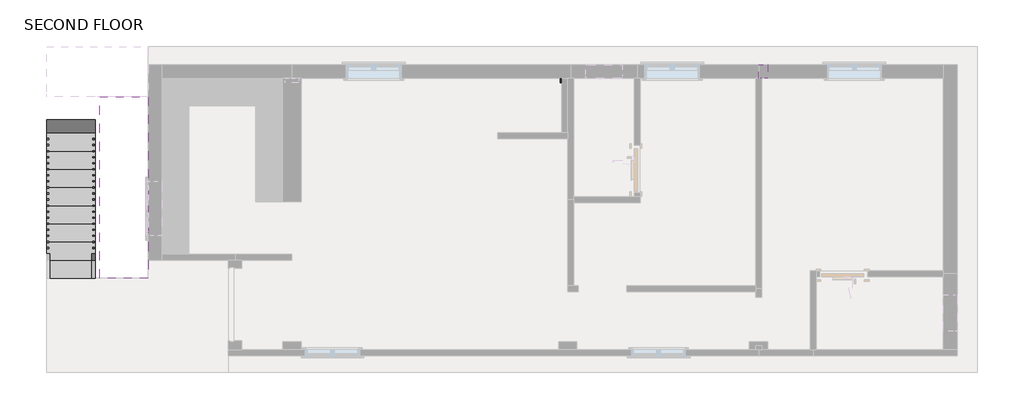
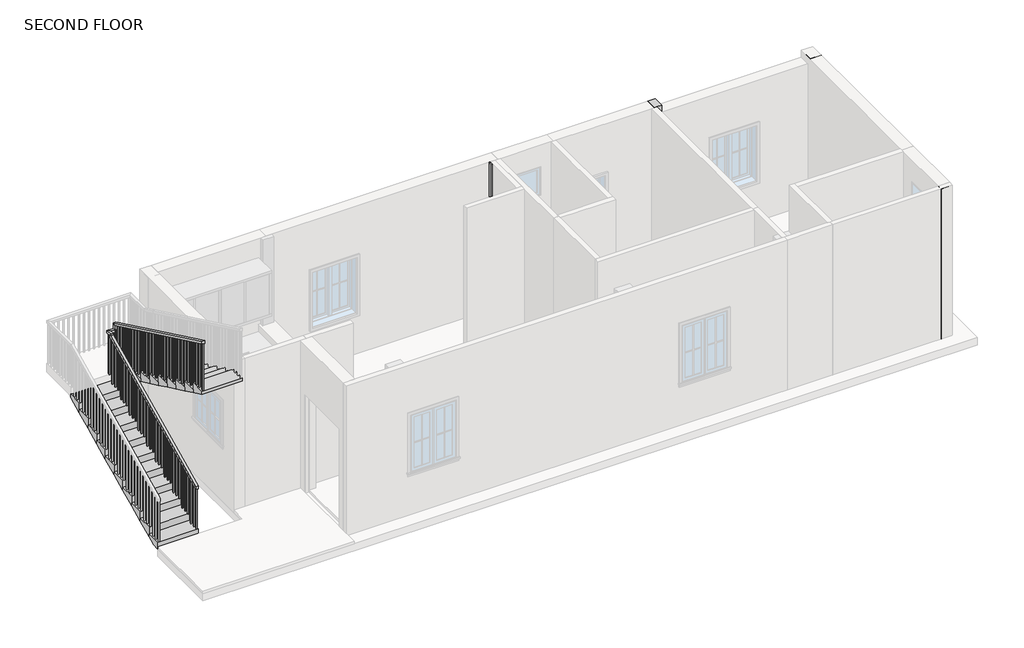
# One storey, part 2 of 3: 4 columns, 2 stair flights, 1 railing.
"""IFC4 building model written with IfcOpenShell, lengths in millimetres."""

from ifc_helpers import new_model, si_unit, frame, origin, place, context, project, spatial, polyline, outline, extrude, faceted_brep, element, save

model = new_model("IFC4")

# Units and contexts
model_context = context("Model", 3, world=origin())
ifc_project = project(units=[si_unit("LENGTHUNIT", "METRE", prefix="MILLI")], contexts=[model_context])

# Site, building, storey
site = spatial("IfcSite", under=ifc_project)
building = spatial("IfcBuilding", under=site)
storey = spatial("IfcBuildingStorey", under=building, Name="SECOND FLOOR", Elevation=6400.8)

# Columns
placement = place(None, origin())
element("IfcColumn", 1, ObjectType="Rectangular Column : 9\" X 12\"", at=placement, inside=storey, context=model_context, shape_type="Brep", body=[
    faceted_brep([(8641.6408773, 5102.5642852, 6400.8), (8870.2408773, 5102.5642852, 6400.8), (8870.2408773, 4797.7642852, 6400.8), (8641.6408773, 4797.7642852, 6400.8), (8641.6408773, 4873.9642852, 6400.8), (8641.6408773, 5102.5642852, 9601.2), (8870.2408773, 5102.5642852, 9601.2), (8641.6408773, 5102.5642852, 9448.8), (8870.2408773, 4797.7642852, 9601.2), (8641.6408773, 4797.7642852, 9601.2)], [[[0, 1, 2, 3, 4]], [[5, 6, 1, 0, 7]], [[6, 8, 2, 1]], [[8, 9, 3, 2]], [[9, 5, 7, 0, 4, 3]], [[5, 9, 8, 6]]]),
])
element("IfcColumn", 2, ObjectType="Rectangular Column : 9\" X 12\"", at=placement, inside=storey, context=model_context, shape_type="Brep", body=[
    faceted_brep([(5695.2408773, 5102.5642852, 9601.2), (5695.2408773, 5102.5642852, 9448.8), (5542.8408773, 5102.5642852, 9448.8), (5542.8408773, 5102.5642852, 9601.2), (5695.2408773, 4873.9642852, 9601.2), (5695.2408773, 4873.9642852, 9448.8), (5593.6408773, 4873.9642852, 9601.2), (5542.8408773, 4873.9642852, 9601.2), (5542.8408773, 4873.9642852, 9448.8)], [[[0, 1, 2, 3]], [[0, 4, 5, 1]], [[5, 4, 6, 7, 8]], [[4, 0, 3, 7, 6]], [[2, 1, 5, 8]], [[3, 2, 8, 7]]]),
])
element("IfcColumn", 3, ObjectType="Rectangular Column : 9\" X 12\"", at=placement, inside=storey, context=model_context, shape_type="SweptSolid", body=[
    extrude(outline(polyline([(2240.8408773, 4797.7642852), (2215.4408773, 4797.7642852), (2215.4408773, 4873.9642852), (2240.8408773, 4873.9642852), (2240.8408773, 4797.7642852)])), frame((0.0, 0.0, 6400.8), z_axis=(0.0, 0.0, 1.0), x_axis=(1.0, 0.0, 0.0)), (0.0, 0.0, 1.0), 3200.4),
])
element("IfcColumn", 4, ObjectType="Rectangular Column : 9\" X 12\"", at=placement, inside=storey, context=model_context, shape_type="SweptSolid", body=[
    extrude(outline(polyline([(8870.2408773, 225.7642852), (8641.6408773, 225.7642852), (8641.6408773, 327.3642852), (8870.2408773, 327.3642852), (8870.2408773, 225.7642852)])), frame((0.0, 0.0, 6400.8), z_axis=(0.0, 0.0, 1.0), x_axis=(1.0, 0.0, 0.0)), (0.0, 0.0, 1.0), 3200.4),
])

# Railing
element("IfcRailing", 5, ObjectType="Handrail - Rectangular", at=placement, inside=storey, context=model_context, shape_type="SolidModel", body=[
    faceted_brep([(-5633.1591227, 1521.1642852, 7460.6727273), (-5633.1591227, 1521.1642852, 7404.3834559), (-5582.3591227, 1521.1642852, 7404.3834559), (-5582.3591227, 1521.1642852, 7460.6727273), (-5633.1591227, 4492.9642852, 8879.0318182), (-5633.1591227, 4543.7642852, 8846.9880014), (-5582.3591227, 4543.7642852, 8846.9880014), (-5582.3591227, 4492.9642852, 8879.0318182), (-5633.1591227, 4492.9642852, 8915.4), (-5633.1591227, 4543.7642852, 8864.6), (-5582.3591227, 4543.7642852, 8864.6), (-5582.3591227, 4492.9642852, 8915.4), (-5633.1591227, 4619.9642852, 8915.4), (-5633.1591227, 4619.9642852, 8864.6), (-5582.3591227, 4569.1642852, 8864.6), (-5582.3591227, 4569.1642852, 8915.4), (-5506.1591227, 4619.9642852, 8915.4), (-5506.1591227, 4619.9642852, 8864.6), (-5506.1591227, 4569.1642852, 8864.6), (-5506.1591227, 4569.1642852, 8915.4), (-5480.7591227, 4619.9642852, 8915.4), (-5480.7591227, 4569.1642852, 8915.4), (-5480.7591227, 4569.1642852, 8864.6), (-5480.7591227, 4619.9642852, 8864.6)], [[[0, 1, 2, 3]], [[1, 0, 4, 5]], [[2, 1, 5, 6]], [[3, 2, 6, 7]], [[0, 3, 7, 4]], [[5, 4, 8, 9]], [[6, 5, 9, 10]], [[7, 6, 10, 11]], [[4, 7, 11, 8]], [[9, 8, 12, 13]], [[10, 9, 13, 14]], [[11, 10, 14, 15]], [[8, 11, 15, 12]], [[13, 12, 16, 17]], [[14, 13, 17, 18]], [[15, 14, 18, 19]], [[12, 15, 19, 16]], [[20, 21, 22, 23]], [[17, 16, 20, 23]], [[18, 17, 23, 22]], [[19, 18, 22, 21]], [[16, 19, 21, 20]]]),
    faceted_brep([(-5506.1591227, 4619.9642852, 8915.4), (-5455.3591227, 4619.9642852, 8864.6), (-5455.3591227, 4569.1642852, 8864.6), (-5506.1591227, 4569.1642852, 8915.4), (-5506.1591227, 4619.9642852, 9036.6272727), (-5506.1591227, 4569.1642852, 9004.5834559), (-5455.3591227, 4569.1642852, 9004.5834559), (-5455.3591227, 4619.9642852, 9036.6272727)], [[[0, 1, 2, 3]], [[4, 5, 6, 7]], [[1, 0, 4, 7]], [[2, 1, 7, 6]], [[3, 2, 6, 5]], [[0, 3, 5, 4]]]),
    faceted_brep([(-5455.3591227, 4619.9642852, 9036.6272727), (-5455.3591227, 4569.1642852, 9004.5834559), (-5506.1591227, 4569.1642852, 9004.5834559), (-5506.1591227, 4619.9642852, 9036.6272727), (-5455.3591227, 1521.1642852, 10515.6), (-5506.1591227, 1521.1642852, 10515.6), (-5506.1591227, 1521.1642852, 10459.3107287), (-5455.3591227, 1521.1642852, 10459.3107287)], [[[0, 1, 2, 3]], [[4, 5, 6, 7]], [[1, 0, 4, 7]], [[2, 1, 7, 6]], [[3, 2, 6, 5]], [[0, 3, 5, 4]]]),
    extrude(outline(polyline([(1537.0392852, 10451.7340241), (1556.0892852, 10442.6419787), (1556.0892852, 9455.7272727), (1537.0392852, 9455.7272727), (1537.0392852, 10451.7340241)])), frame((-5490.2841227, 0.0, 0.0), z_axis=(1.0, 0.0, 0.0), x_axis=(0.0, 1.0, 0.0)), (0.0, 0.0, 1.0), 19.05),
    extrude(outline(polyline([(1638.6392852, 10403.243115), (1657.6892852, 10394.1510696), (1657.6892852, 9455.7272727), (1638.6392852, 9455.7272727), (1638.6392852, 10403.243115)])), frame((-5490.2841227, 0.0, 0.0), z_axis=(1.0, 0.0, 0.0), x_axis=(0.0, 1.0, 0.0)), (0.0, 0.0, 1.0), 19.05),
    extrude(outline(polyline([(1740.2392852, 10354.7522059), (1759.2892852, 10345.6601605), (1759.2892852, 9455.7272727), (1740.2392852, 9455.7272727), (1740.2392852, 10354.7522059)])), frame((-5490.2841227, 0.0, 0.0), z_axis=(1.0, 0.0, 0.0), x_axis=(0.0, 1.0, 0.0)), (0.0, 0.0, 1.0), 19.05),
    extrude(outline(polyline([(1841.8392852, 10306.2612969), (1860.8892852, 10297.1692514), (1860.8892852, 9310.2545455), (1841.8392852, 9310.2545455), (1841.8392852, 10306.2612969)])), frame((-5490.2841227, 0.0, 0.0), z_axis=(1.0, 0.0, 0.0), x_axis=(0.0, 1.0, 0.0)), (0.0, 0.0, 1.0), 19.05),
    extrude(outline(polyline([(1943.4392852, 10257.7703878), (1962.4892852, 10248.6783423), (1962.4892852, 9310.2545455), (1943.4392852, 9310.2545455), (1943.4392852, 10257.7703878)])), frame((-5490.2841227, 0.0, 0.0), z_axis=(1.0, 0.0, 0.0), x_axis=(0.0, 1.0, 0.0)), (0.0, 0.0, 1.0), 19.05),
    extrude(outline(polyline([(2045.0392852, 10209.2794787), (2064.0892852, 10200.1874332), (2064.0892852, 9310.2545455), (2045.0392852, 9310.2545455), (2045.0392852, 10209.2794787)])), frame((-5490.2841227, 0.0, 0.0), z_axis=(1.0, 0.0, 0.0), x_axis=(0.0, 1.0, 0.0)), (0.0, 0.0, 1.0), 19.05),
    extrude(outline(polyline([(2146.6392852, 10160.7885696), (2165.6892852, 10151.6965241), (2165.6892852, 9164.7818182), (2146.6392852, 9164.7818182), (2146.6392852, 10160.7885696)])), frame((-5490.2841227, 0.0, 0.0), z_axis=(1.0, 0.0, 0.0), x_axis=(0.0, 1.0, 0.0)), (0.0, 0.0, 1.0), 19.05),
    extrude(outline(polyline([(2248.2392852, 10112.2976605), (2267.2892852, 10103.205615), (2267.2892852, 9164.7818182), (2248.2392852, 9164.7818182), (2248.2392852, 10112.2976605)])), frame((-5490.2841227, 0.0, 0.0), z_axis=(1.0, 0.0, 0.0), x_axis=(0.0, 1.0, 0.0)), (0.0, 0.0, 1.0), 19.05),
    extrude(outline(polyline([(2349.8392852, 10063.8067514), (2368.8892852, 10054.7147059), (2368.8892852, 9164.7818182), (2349.8392852, 9164.7818182), (2349.8392852, 10063.8067514)])), frame((-5490.2841227, 0.0, 0.0), z_axis=(1.0, 0.0, 0.0), x_axis=(0.0, 1.0, 0.0)), (0.0, 0.0, 1.0), 19.05),
    extrude(outline(polyline([(2451.4392852, 10015.3158423), (2470.4892852, 10006.2237969), (2470.4892852, 9019.3090909), (2451.4392852, 9019.3090909), (2451.4392852, 10015.3158423)])), frame((-5490.2841227, 0.0, 0.0), z_axis=(1.0, 0.0, 0.0), x_axis=(0.0, 1.0, 0.0)), (0.0, 0.0, 1.0), 19.05),
    extrude(outline(polyline([(2553.0392852, 9966.8249332), (2572.0892852, 9957.7328878), (2572.0892852, 9019.3090909), (2553.0392852, 9019.3090909), (2553.0392852, 9966.8249332)])), frame((-5490.2841227, 0.0, 0.0), z_axis=(1.0, 0.0, 0.0), x_axis=(0.0, 1.0, 0.0)), (0.0, 0.0, 1.0), 19.05),
    extrude(outline(polyline([(2654.6392852, 9918.3340241), (2673.6892852, 9909.2419787), (2673.6892852, 9019.3090909), (2654.6392852, 9019.3090909), (2654.6392852, 9918.3340241)])), frame((-5490.2841227, 0.0, 0.0), z_axis=(1.0, 0.0, 0.0), x_axis=(0.0, 1.0, 0.0)), (0.0, 0.0, 1.0), 19.05),
    extrude(outline(polyline([(2756.2392852, 9869.843115), (2775.2892852, 9860.7510696), (2775.2892852, 8873.8363636), (2756.2392852, 8873.8363636), (2756.2392852, 9869.843115)])), frame((-5490.2841227, 0.0, 0.0), z_axis=(1.0, 0.0, 0.0), x_axis=(0.0, 1.0, 0.0)), (0.0, 0.0, 1.0), 19.05),
    extrude(outline(polyline([(2857.8392852, 9821.3522059), (2876.8892852, 9812.2601605), (2876.8892852, 8873.8363636), (2857.8392852, 8873.8363636), (2857.8392852, 9821.3522059)])), frame((-5490.2841227, 0.0, 0.0), z_axis=(1.0, 0.0, 0.0), x_axis=(0.0, 1.0, 0.0)), (0.0, 0.0, 1.0), 19.05),
    extrude(outline(polyline([(2959.4392852, 9772.8612969), (2978.4892852, 9763.7692514), (2978.4892852, 8873.8363636), (2959.4392852, 8873.8363636), (2959.4392852, 9772.8612969)])), frame((-5490.2841227, 0.0, 0.0), z_axis=(1.0, 0.0, 0.0), x_axis=(0.0, 1.0, 0.0)), (0.0, 0.0, 1.0), 19.05),
    extrude(outline(polyline([(3061.0392852, 9724.3703878), (3080.0892852, 9715.2783423), (3080.0892852, 8728.3636364), (3061.0392852, 8728.3636364), (3061.0392852, 9724.3703878)])), frame((-5490.2841227, 0.0, 0.0), z_axis=(1.0, 0.0, 0.0), x_axis=(0.0, 1.0, 0.0)), (0.0, 0.0, 1.0), 19.05),
    extrude(outline(polyline([(3162.6392852, 9675.8794787), (3181.6892852, 9666.7874332), (3181.6892852, 8728.3636364), (3162.6392852, 8728.3636364), (3162.6392852, 9675.8794787)])), frame((-5490.2841227, 0.0, 0.0), z_axis=(1.0, 0.0, 0.0), x_axis=(0.0, 1.0, 0.0)), (0.0, 0.0, 1.0), 19.05),
    extrude(outline(polyline([(3264.2392852, 9627.3885696), (3283.2892852, 9618.2965241), (3283.2892852, 8728.3636364), (3264.2392852, 8728.3636364), (3264.2392852, 9627.3885696)])), frame((-5490.2841227, 0.0, 0.0), z_axis=(1.0, 0.0, 0.0), x_axis=(0.0, 1.0, 0.0)), (0.0, 0.0, 1.0), 19.05),
    extrude(outline(polyline([(3365.8392852, 9578.8976605), (3384.8892852, 9569.805615), (3384.8892852, 8582.8909091), (3365.8392852, 8582.8909091), (3365.8392852, 9578.8976605)])), frame((-5490.2841227, 0.0, 0.0), z_axis=(1.0, 0.0, 0.0), x_axis=(0.0, 1.0, 0.0)), (0.0, 0.0, 1.0), 19.05),
    extrude(outline(polyline([(3467.4392852, 9530.4067514), (3486.4892852, 9521.3147059), (3486.4892852, 8582.8909091), (3467.4392852, 8582.8909091), (3467.4392852, 9530.4067514)])), frame((-5490.2841227, 0.0, 0.0), z_axis=(1.0, 0.0, 0.0), x_axis=(0.0, 1.0, 0.0)), (0.0, 0.0, 1.0), 19.05),
    extrude(outline(polyline([(3569.0392852, 9481.9158423), (3588.0892852, 9472.8237969), (3588.0892852, 8582.8909091), (3569.0392852, 8582.8909091), (3569.0392852, 9481.9158423)])), frame((-5490.2841227, 0.0, 0.0), z_axis=(1.0, 0.0, 0.0), x_axis=(0.0, 1.0, 0.0)), (0.0, 0.0, 1.0), 19.05),
    extrude(outline(polyline([(3670.6392852, 9433.4249332), (3689.6892852, 9424.3328878), (3689.6892852, 8437.4181818), (3670.6392852, 8437.4181818), (3670.6392852, 9433.4249332)])), frame((-5490.2841227, 0.0, 0.0), z_axis=(1.0, 0.0, 0.0), x_axis=(0.0, 1.0, 0.0)), (0.0, 0.0, 1.0), 19.05),
    extrude(outline(polyline([(3772.2392852, 9384.9340241), (3791.2892852, 9375.8419787), (3791.2892852, 8437.4181818), (3772.2392852, 8437.4181818), (3772.2392852, 9384.9340241)])), frame((-5490.2841227, 0.0, 0.0), z_axis=(1.0, 0.0, 0.0), x_axis=(0.0, 1.0, 0.0)), (0.0, 0.0, 1.0), 19.05),
    extrude(outline(polyline([(3873.8392852, 9336.443115), (3892.8892852, 9327.3510696), (3892.8892852, 8437.4181818), (3873.8392852, 8437.4181818), (3873.8392852, 9336.443115)])), frame((-5490.2841227, 0.0, 0.0), z_axis=(1.0, 0.0, 0.0), x_axis=(0.0, 1.0, 0.0)), (0.0, 0.0, 1.0), 19.05),
    extrude(outline(polyline([(3975.4392852, 9287.9522059), (3994.4892852, 9278.8601605), (3994.4892852, 8291.9454545), (3975.4392852, 8291.9454545), (3975.4392852, 9287.9522059)])), frame((-5490.2841227, 0.0, 0.0), z_axis=(1.0, 0.0, 0.0), x_axis=(0.0, 1.0, 0.0)), (0.0, 0.0, 1.0), 19.05),
    extrude(outline(polyline([(4077.0392852, 9239.4612969), (4096.0892852, 9230.3692514), (4096.0892852, 8291.9454545), (4077.0392852, 8291.9454545), (4077.0392852, 9239.4612969)])), frame((-5490.2841227, 0.0, 0.0), z_axis=(1.0, 0.0, 0.0), x_axis=(0.0, 1.0, 0.0)), (0.0, 0.0, 1.0), 19.05),
    extrude(outline(polyline([(4178.6392852, 9190.9703878), (4197.6892852, 9181.8783423), (4197.6892852, 8291.9454545), (4178.6392852, 8291.9454545), (4178.6392852, 9190.9703878)])), frame((-5490.2841227, 0.0, 0.0), z_axis=(1.0, 0.0, 0.0), x_axis=(0.0, 1.0, 0.0)), (0.0, 0.0, 1.0), 19.05),
    extrude(outline(polyline([(4280.2392852, 9142.4794787), (4299.2892852, 9133.3874332), (4299.2892852, 8146.4727273), (4280.2392852, 8146.4727273), (4280.2392852, 9142.4794787)])), frame((-5490.2841227, 0.0, 0.0), z_axis=(1.0, 0.0, 0.0), x_axis=(0.0, 1.0, 0.0)), (0.0, 0.0, 1.0), 19.05),
    extrude(outline(polyline([(4381.8392852, 9093.9885696), (4400.8892852, 9084.8965241), (4400.8892852, 8146.4727273), (4381.8392852, 8146.4727273), (4381.8392852, 9093.9885696)])), frame((-5490.2841227, 0.0, 0.0), z_axis=(1.0, 0.0, 0.0), x_axis=(0.0, 1.0, 0.0)), (0.0, 0.0, 1.0), 19.05),
    extrude(outline(polyline([(4483.4392852, 9045.4976605), (4502.4892852, 9036.405615), (4502.4892852, 8146.4727273), (4483.4392852, 8146.4727273), (4483.4392852, 9045.4976605)])), frame((-5490.2841227, 0.0, 0.0), z_axis=(1.0, 0.0, 0.0), x_axis=(0.0, 1.0, 0.0)), (0.0, 0.0, 1.0), 19.05),
    extrude(outline(polyline([(-5515.6841227, 4585.0392852), (-5515.6841227, 4604.0892852), (-5496.6341227, 4604.0892852), (-5496.6341227, 4585.0392852), (-5515.6841227, 4585.0392852)])), frame((0.0, 0.0, 8001.0), z_axis=(0.0, 0.0, 1.0), x_axis=(1.0, 0.0, 0.0)), (0.0, 0.0, 1.0), 863.6),
    extrude(outline(polyline([(-5598.2341227, 4559.6392852), (-5617.2841227, 4559.6392852), (-5617.2841227, 4578.6892852), (-5598.2341227, 4578.6892852), (-5598.2341227, 4559.6392852)])), frame((0.0, 0.0, 8001.0), z_axis=(0.0, 0.0, 1.0), x_axis=(1.0, 0.0, 0.0)), (0.0, 0.0, 1.0), 863.6),
    extrude(outline(polyline([(4458.0392852, 8806.0737969), (4477.0892852, 8815.1658423), (4477.0892852, 7855.5272727), (4458.0392852, 7855.5272727), (4458.0392852, 8806.0737969)])), frame((-5617.2841227, 0.0, 0.0), z_axis=(1.0, 0.0, 0.0), x_axis=(0.0, 1.0, 0.0)), (0.0, 0.0, 1.0), 19.05),
    extrude(outline(polyline([(4356.4392852, 8757.5828878), (4375.4892852, 8766.6749332), (4375.4892852, 7855.5272727), (4356.4392852, 7855.5272727), (4356.4392852, 8757.5828878)])), frame((-5617.2841227, 0.0, 0.0), z_axis=(1.0, 0.0, 0.0), x_axis=(0.0, 1.0, 0.0)), (0.0, 0.0, 1.0), 19.05),
    extrude(outline(polyline([(4254.8392852, 8709.0919787), (4273.8892852, 8718.1840241), (4273.8892852, 7855.5272727), (4254.8392852, 7855.5272727), (4254.8392852, 8709.0919787)])), frame((-5617.2841227, 0.0, 0.0), z_axis=(1.0, 0.0, 0.0), x_axis=(0.0, 1.0, 0.0)), (0.0, 0.0, 1.0), 19.05),
    extrude(outline(polyline([(4153.2392852, 8660.6010696), (4172.2892852, 8669.693115), (4172.2892852, 7710.0545455), (4153.2392852, 7710.0545455), (4153.2392852, 8660.6010696)])), frame((-5617.2841227, 0.0, 0.0), z_axis=(1.0, 0.0, 0.0), x_axis=(0.0, 1.0, 0.0)), (0.0, 0.0, 1.0), 19.05),
    extrude(outline(polyline([(4051.6392852, 8612.1101605), (4070.6892852, 8621.2022059), (4070.6892852, 7710.0545455), (4051.6392852, 7710.0545455), (4051.6392852, 8612.1101605)])), frame((-5617.2841227, 0.0, 0.0), z_axis=(1.0, 0.0, 0.0), x_axis=(0.0, 1.0, 0.0)), (0.0, 0.0, 1.0), 19.05),
    extrude(outline(polyline([(3950.0392852, 8563.6192514), (3969.0892852, 8572.7112969), (3969.0892852, 7710.0545455), (3950.0392852, 7710.0545455), (3950.0392852, 8563.6192514)])), frame((-5617.2841227, 0.0, 0.0), z_axis=(1.0, 0.0, 0.0), x_axis=(0.0, 1.0, 0.0)), (0.0, 0.0, 1.0), 19.05),
    extrude(outline(polyline([(3848.4392852, 8515.1283423), (3867.4892852, 8524.2203878), (3867.4892852, 7564.5818182), (3848.4392852, 7564.5818182), (3848.4392852, 8515.1283423)])), frame((-5617.2841227, 0.0, 0.0), z_axis=(1.0, 0.0, 0.0), x_axis=(0.0, 1.0, 0.0)), (0.0, 0.0, 1.0), 19.05),
    extrude(outline(polyline([(3746.8392852, 8466.6374332), (3765.8892852, 8475.7294787), (3765.8892852, 7564.5818182), (3746.8392852, 7564.5818182), (3746.8392852, 8466.6374332)])), frame((-5617.2841227, 0.0, 0.0), z_axis=(1.0, 0.0, 0.0), x_axis=(0.0, 1.0, 0.0)), (0.0, 0.0, 1.0), 19.05),
    extrude(outline(polyline([(3645.2392852, 8418.1465241), (3664.2892852, 8427.2385696), (3664.2892852, 7564.5818182), (3645.2392852, 7564.5818182), (3645.2392852, 8418.1465241)])), frame((-5617.2841227, 0.0, 0.0), z_axis=(1.0, 0.0, 0.0), x_axis=(0.0, 1.0, 0.0)), (0.0, 0.0, 1.0), 19.05),
    extrude(outline(polyline([(3543.6392852, 8369.655615), (3562.6892852, 8378.7476605), (3562.6892852, 7419.1090909), (3543.6392852, 7419.1090909), (3543.6392852, 8369.655615)])), frame((-5617.2841227, 0.0, 0.0), z_axis=(1.0, 0.0, 0.0), x_axis=(0.0, 1.0, 0.0)), (0.0, 0.0, 1.0), 19.05),
    extrude(outline(polyline([(3442.0392852, 8321.1647059), (3461.0892852, 8330.2567514), (3461.0892852, 7419.1090909), (3442.0392852, 7419.1090909), (3442.0392852, 8321.1647059)])), frame((-5617.2841227, 0.0, 0.0), z_axis=(1.0, 0.0, 0.0), x_axis=(0.0, 1.0, 0.0)), (0.0, 0.0, 1.0), 19.05),
    extrude(outline(polyline([(3340.4392852, 8272.6737969), (3359.4892852, 8281.7658423), (3359.4892852, 7419.1090909), (3340.4392852, 7419.1090909), (3340.4392852, 8272.6737969)])), frame((-5617.2841227, 0.0, 0.0), z_axis=(1.0, 0.0, 0.0), x_axis=(0.0, 1.0, 0.0)), (0.0, 0.0, 1.0), 19.05),
    extrude(outline(polyline([(3238.8392852, 8224.1828878), (3257.8892852, 8233.2749332), (3257.8892852, 7273.6363636), (3238.8392852, 7273.6363636), (3238.8392852, 8224.1828878)])), frame((-5617.2841227, 0.0, 0.0), z_axis=(1.0, 0.0, 0.0), x_axis=(0.0, 1.0, 0.0)), (0.0, 0.0, 1.0), 19.05),
    extrude(outline(polyline([(3137.2392852, 8175.6919787), (3156.2892852, 8184.7840241), (3156.2892852, 7273.6363636), (3137.2392852, 7273.6363636), (3137.2392852, 8175.6919787)])), frame((-5617.2841227, 0.0, 0.0), z_axis=(1.0, 0.0, 0.0), x_axis=(0.0, 1.0, 0.0)), (0.0, 0.0, 1.0), 19.05),
    extrude(outline(polyline([(3035.6392852, 8127.2010696), (3054.6892852, 8136.293115), (3054.6892852, 7273.6363636), (3035.6392852, 7273.6363636), (3035.6392852, 8127.2010696)])), frame((-5617.2841227, 0.0, 0.0), z_axis=(1.0, 0.0, 0.0), x_axis=(0.0, 1.0, 0.0)), (0.0, 0.0, 1.0), 19.05),
    extrude(outline(polyline([(2934.0392852, 8078.7101605), (2953.0892852, 8087.8022059), (2953.0892852, 7128.1636364), (2934.0392852, 7128.1636364), (2934.0392852, 8078.7101605)])), frame((-5617.2841227, 0.0, 0.0), z_axis=(1.0, 0.0, 0.0), x_axis=(0.0, 1.0, 0.0)), (0.0, 0.0, 1.0), 19.05),
    extrude(outline(polyline([(2832.4392852, 8030.2192514), (2851.4892852, 8039.3112969), (2851.4892852, 7128.1636364), (2832.4392852, 7128.1636364), (2832.4392852, 8030.2192514)])), frame((-5617.2841227, 0.0, 0.0), z_axis=(1.0, 0.0, 0.0), x_axis=(0.0, 1.0, 0.0)), (0.0, 0.0, 1.0), 19.05),
    extrude(outline(polyline([(2730.8392852, 7981.7283423), (2749.8892852, 7990.8203878), (2749.8892852, 7128.1636364), (2730.8392852, 7128.1636364), (2730.8392852, 7981.7283423)])), frame((-5617.2841227, 0.0, 0.0), z_axis=(1.0, 0.0, 0.0), x_axis=(0.0, 1.0, 0.0)), (0.0, 0.0, 1.0), 19.05),
    extrude(outline(polyline([(2629.2392852, 7933.2374332), (2648.2892852, 7942.3294787), (2648.2892852, 6982.6909091), (2629.2392852, 6982.6909091), (2629.2392852, 7933.2374332)])), frame((-5617.2841227, 0.0, 0.0), z_axis=(1.0, 0.0, 0.0), x_axis=(0.0, 1.0, 0.0)), (0.0, 0.0, 1.0), 19.05),
    extrude(outline(polyline([(2527.6392852, 7884.7465241), (2546.6892852, 7893.8385696), (2546.6892852, 6982.6909091), (2527.6392852, 6982.6909091), (2527.6392852, 7884.7465241)])), frame((-5617.2841227, 0.0, 0.0), z_axis=(1.0, 0.0, 0.0), x_axis=(0.0, 1.0, 0.0)), (0.0, 0.0, 1.0), 19.05),
    extrude(outline(polyline([(2426.0392852, 7836.255615), (2445.0892852, 7845.3476605), (2445.0892852, 6982.6909091), (2426.0392852, 6982.6909091), (2426.0392852, 7836.255615)])), frame((-5617.2841227, 0.0, 0.0), z_axis=(1.0, 0.0, 0.0), x_axis=(0.0, 1.0, 0.0)), (0.0, 0.0, 1.0), 19.05),
    extrude(outline(polyline([(2324.4392852, 7787.7647059), (2343.4892852, 7796.8567514), (2343.4892852, 6837.2181818), (2324.4392852, 6837.2181818), (2324.4392852, 7787.7647059)])), frame((-5617.2841227, 0.0, 0.0), z_axis=(1.0, 0.0, 0.0), x_axis=(0.0, 1.0, 0.0)), (0.0, 0.0, 1.0), 19.05),
    extrude(outline(polyline([(2222.8392852, 7739.2737969), (2241.8892852, 7748.3658423), (2241.8892852, 6837.2181818), (2222.8392852, 6837.2181818), (2222.8392852, 7739.2737969)])), frame((-5617.2841227, 0.0, 0.0), z_axis=(1.0, 0.0, 0.0), x_axis=(0.0, 1.0, 0.0)), (0.0, 0.0, 1.0), 19.05),
    extrude(outline(polyline([(2121.2392852, 7690.7828878), (2140.2892852, 7699.8749332), (2140.2892852, 6837.2181818), (2121.2392852, 6837.2181818), (2121.2392852, 7690.7828878)])), frame((-5617.2841227, 0.0, 0.0), z_axis=(1.0, 0.0, 0.0), x_axis=(0.0, 1.0, 0.0)), (0.0, 0.0, 1.0), 19.05),
    extrude(outline(polyline([(2019.6392852, 7642.2919787), (2038.6892852, 7651.3840241), (2038.6892852, 6691.7454545), (2019.6392852, 6691.7454545), (2019.6392852, 7642.2919787)])), frame((-5617.2841227, 0.0, 0.0), z_axis=(1.0, 0.0, 0.0), x_axis=(0.0, 1.0, 0.0)), (0.0, 0.0, 1.0), 19.05),
    extrude(outline(polyline([(1918.0392852, 7593.8010696), (1937.0892852, 7602.893115), (1937.0892852, 6691.7454545), (1918.0392852, 6691.7454545), (1918.0392852, 7593.8010696)])), frame((-5617.2841227, 0.0, 0.0), z_axis=(1.0, 0.0, 0.0), x_axis=(0.0, 1.0, 0.0)), (0.0, 0.0, 1.0), 19.05),
    extrude(outline(polyline([(1816.4392852, 7545.3101605), (1835.4892852, 7554.4022059), (1835.4892852, 6691.7454545), (1816.4392852, 6691.7454545), (1816.4392852, 7545.3101605)])), frame((-5617.2841227, 0.0, 0.0), z_axis=(1.0, 0.0, 0.0), x_axis=(0.0, 1.0, 0.0)), (0.0, 0.0, 1.0), 19.05),
    extrude(outline(polyline([(1714.8392852, 7496.8192514), (1733.8892852, 7505.9112969), (1733.8892852, 6546.2727273), (1714.8392852, 6546.2727273), (1714.8392852, 7496.8192514)])), frame((-5617.2841227, 0.0, 0.0), z_axis=(1.0, 0.0, 0.0), x_axis=(0.0, 1.0, 0.0)), (0.0, 0.0, 1.0), 19.05),
    extrude(outline(polyline([(1613.2392852, 7448.3283423), (1632.2892852, 7457.4203878), (1632.2892852, 6546.2727273), (1613.2392852, 6546.2727273), (1613.2392852, 7448.3283423)])), frame((-5617.2841227, 0.0, 0.0), z_axis=(1.0, 0.0, 0.0), x_axis=(0.0, 1.0, 0.0)), (0.0, 0.0, 1.0), 19.05),
    extrude(outline(polyline([(-5490.2841227, 4585.0392852), (-5490.2841227, 4604.0892852), (-5471.2341227, 4604.0892852), (-5471.2341227, 4585.0392852), (-5490.2841227, 4585.0392852)])), frame((0.0, 0.0, 8001.0), z_axis=(0.0, 0.0, 1.0), x_axis=(1.0, 0.0, 0.0)), (0.0, 0.0, 1.0), 863.6),
    extrude(outline(polyline([(-5598.2341227, 4585.0392852), (-5617.2841227, 4585.0392852), (-5617.2841227, 4604.0892852), (-5598.2341227, 4604.0892852), (-5598.2341227, 4585.0392852)])), frame((0.0, 0.0, 8001.0), z_axis=(0.0, 0.0, 1.0), x_axis=(1.0, 0.0, 0.0)), (0.0, 0.0, 1.0), 863.6),
    extrude(outline(polyline([(1521.1642852, 10459.3107287), (1540.2142852, 10450.2186832), (1540.2142852, 9455.7272727), (1521.1642852, 9455.7272727), (1521.1642852, 10459.3107287)])), frame((-5490.2841227, 0.0, 0.0), z_axis=(1.0, 0.0, 0.0), x_axis=(0.0, 1.0, 0.0)), (0.0, 0.0, 1.0), 19.05),
    extrude(outline(polyline([(1521.1642852, 7404.3834559), (1540.2142852, 7413.4755014), (1540.2142852, 6546.2727273), (1521.1642852, 6546.2727273), (1521.1642852, 7404.3834559)])), frame((-5617.2841227, 0.0, 0.0), z_axis=(1.0, 0.0, 0.0), x_axis=(0.0, 1.0, 0.0)), (0.0, 0.0, 1.0), 19.05),
])

# Stair flights
element("IfcStairFlight", 6, ObjectType="3/4\" Nosing", at=placement, inside=storey, context=model_context, shape_type="Brep", body=[
    faceted_brep([(-6395.1591227, 1825.9642852, 6546.2727273), (-6395.1591227, 1521.1642852, 6546.2727273), (-5582.3591227, 1521.1642852, 6546.2727273), (-5582.3591227, 1825.9642852, 6546.2727273), (-6395.1591227, 1825.9642852, 6475.9111381), (-6395.1591227, 1668.5885672, 6400.8), (-6395.1591227, 1521.1642852, 6400.8), (-5582.3591227, 1521.1642852, 6400.8), (-5582.3591227, 1668.5885672, 6400.8), (-5582.3591227, 1825.9642852, 6475.9111381), (-6395.1591227, 2130.7642852, 6691.7454545), (-6395.1591227, 1825.9642852, 6691.7454545), (-5582.3591227, 1825.9642852, 6691.7454545), (-5582.3591227, 2130.7642852, 6691.7454545), (-6395.1591227, 2130.7642852, 6621.3838654), (-5582.3591227, 2130.7642852, 6621.3838654), (-6395.1591227, 2435.5642852, 6837.2181818), (-6395.1591227, 2130.7642852, 6837.2181818), (-5582.3591227, 2130.7642852, 6837.2181818), (-5582.3591227, 2435.5642852, 6837.2181818), (-6395.1591227, 2435.5642852, 6766.8565927), (-5582.3591227, 2435.5642852, 6766.8565927), (-6395.1591227, 2740.3642852, 6982.6909091), (-6395.1591227, 2435.5642852, 6982.6909091), (-5582.3591227, 2435.5642852, 6982.6909091), (-5582.3591227, 2740.3642852, 6982.6909091), (-6395.1591227, 2740.3642852, 6912.3293199), (-5582.3591227, 2740.3642852, 6912.3293199), (-6395.1591227, 3045.1642852, 7128.1636364), (-6395.1591227, 2740.3642852, 7128.1636364), (-5582.3591227, 2740.3642852, 7128.1636364), (-5582.3591227, 3045.1642852, 7128.1636364), (-6395.1591227, 3045.1642852, 7057.8020472), (-5582.3591227, 3045.1642852, 7057.8020472), (-6395.1591227, 3349.9642852, 7273.6363636), (-6395.1591227, 3045.1642852, 7273.6363636), (-5582.3591227, 3045.1642852, 7273.6363636), (-5582.3591227, 3349.9642852, 7273.6363636), (-6395.1591227, 3349.9642852, 7203.2747745), (-5582.3591227, 3349.9642852, 7203.2747745), (-6395.1591227, 3654.7642852, 7419.1090909), (-6395.1591227, 3349.9642852, 7419.1090909), (-5582.3591227, 3349.9642852, 7419.1090909), (-5582.3591227, 3654.7642852, 7419.1090909), (-6395.1591227, 3654.7642852, 7348.7475018), (-5582.3591227, 3654.7642852, 7348.7475018), (-6395.1591227, 3959.5642852, 7564.5818182), (-6395.1591227, 3654.7642852, 7564.5818182), (-5582.3591227, 3654.7642852, 7564.5818182), (-5582.3591227, 3959.5642852, 7564.5818182), (-6395.1591227, 3959.5642852, 7494.220229), (-5582.3591227, 3959.5642852, 7494.220229), (-6395.1591227, 4264.3642852, 7639.6929563), (-6395.1591227, 4569.1642852, 7785.1656836), (-5582.3591227, 4569.1642852, 7785.1656836), (-5582.3591227, 4264.3642852, 7639.6929563), (-6395.1591227, 4264.3642852, 7710.0545455), (-6395.1591227, 3959.5642852, 7710.0545455), (-5582.3591227, 3959.5642852, 7710.0545455), (-5582.3591227, 4264.3642852, 7710.0545455), (-6395.1591227, 4569.1642852, 7855.5272727), (-6395.1591227, 4264.3642852, 7855.5272727), (-5582.3591227, 4264.3642852, 7855.5272727), (-5582.3591227, 4569.1642852, 7855.5272727), (-5582.3591227, 4569.1642852, 7823.2)], [[[0, 1, 2, 3]], [[1, 0, 4, 5, 6]], [[2, 1, 6, 7]], [[3, 2, 7, 8, 9]], [[10, 11, 12, 13]], [[11, 10, 14, 4, 0]], [[0, 3, 12, 11]], [[13, 12, 3, 9, 15]], [[16, 17, 18, 19]], [[17, 16, 20, 14, 10]], [[10, 13, 18, 17]], [[19, 18, 13, 15, 21]], [[22, 23, 24, 25]], [[23, 22, 26, 20, 16]], [[16, 19, 24, 23]], [[25, 24, 19, 21, 27]], [[28, 29, 30, 31]], [[29, 28, 32, 26, 22]], [[22, 25, 30, 29]], [[31, 30, 25, 27, 33]], [[34, 35, 36, 37]], [[35, 34, 38, 32, 28]], [[28, 31, 36, 35]], [[37, 36, 31, 33, 39]], [[40, 41, 42, 43]], [[41, 40, 44, 38, 34]], [[34, 37, 42, 41]], [[43, 42, 37, 39, 45]], [[46, 47, 48, 49]], [[47, 46, 50, 44, 40]], [[40, 43, 48, 47]], [[49, 48, 43, 45, 51]], [[7, 6, 5, 8]], [[8, 5, 4, 14, 20, 26, 32, 38, 44, 50, 52, 53, 54, 55, 51, 45, 39, 33, 27, 21, 15, 9]], [[56, 57, 58, 59]], [[57, 56, 52, 50, 46]], [[46, 49, 58, 57]], [[59, 58, 49, 51, 55]], [[60, 61, 62, 63]], [[61, 60, 53, 52, 56]], [[56, 59, 62, 61]], [[63, 62, 59, 55, 54, 64]], [[60, 63, 64, 54, 53]]]),
])
element("IfcStairFlight", 7, ObjectType="3/4\" Nosing", at=placement, inside=storey, context=model_context, shape_type="Brep", body=[
    faceted_brep([(-4693.3591227, 4264.3642852, 8146.4727273), (-4693.3591227, 4569.1642852, 8146.4727273), (-5506.1591227, 4569.1642852, 8146.4727273), (-5506.1591227, 4264.3642852, 8146.4727273), (-4693.3591227, 4264.3642852, 8076.1111381), (-4693.3591227, 4569.1642852, 7930.6384108), (-4693.3591227, 4569.1642852, 8001.0), (-5506.1591227, 4569.1642852, 7930.6384108), (-5506.1591227, 4264.3642852, 8076.1111381), (-4693.3591227, 3959.5642852, 8291.9454545), (-4693.3591227, 4264.3642852, 8291.9454545), (-5506.1591227, 4264.3642852, 8291.9454545), (-5506.1591227, 3959.5642852, 8291.9454545), (-4693.3591227, 3959.5642852, 8221.5838654), (-5506.1591227, 3959.5642852, 8221.5838654), (-4693.3591227, 3654.7642852, 8437.4181818), (-4693.3591227, 3959.5642852, 8437.4181818), (-5506.1591227, 3959.5642852, 8437.4181818), (-5506.1591227, 3654.7642852, 8437.4181818), (-4693.3591227, 3654.7642852, 8367.0565927), (-5506.1591227, 3654.7642852, 8367.0565927), (-4693.3591227, 3349.9642852, 8582.8909091), (-4693.3591227, 3654.7642852, 8582.8909091), (-5506.1591227, 3654.7642852, 8582.8909091), (-5506.1591227, 3349.9642852, 8582.8909091), (-4693.3591227, 3349.9642852, 8512.5293199), (-5506.1591227, 3349.9642852, 8512.5293199), (-4693.3591227, 3045.1642852, 8728.3636364), (-4693.3591227, 3349.9642852, 8728.3636364), (-5506.1591227, 3349.9642852, 8728.3636364), (-5506.1591227, 3045.1642852, 8728.3636364), (-4693.3591227, 3045.1642852, 8658.0020472), (-5506.1591227, 3045.1642852, 8658.0020472), (-4693.3591227, 2740.3642852, 8873.8363636), (-4693.3591227, 3045.1642852, 8873.8363636), (-5506.1591227, 3045.1642852, 8873.8363636), (-5506.1591227, 2740.3642852, 8873.8363636), (-4693.3591227, 2740.3642852, 8803.4747745), (-5506.1591227, 2740.3642852, 8803.4747745), (-4693.3591227, 2435.5642852, 9019.3090909), (-4693.3591227, 2740.3642852, 9019.3090909), (-5506.1591227, 2740.3642852, 9019.3090909), (-5506.1591227, 2435.5642852, 9019.3090909), (-4693.3591227, 2435.5642852, 8948.9475018), (-5506.1591227, 2435.5642852, 8948.9475018), (-4693.3591227, 2130.7642852, 9164.7818182), (-4693.3591227, 2435.5642852, 9164.7818182), (-5506.1591227, 2435.5642852, 9164.7818182), (-5506.1591227, 2130.7642852, 9164.7818182), (-4693.3591227, 2130.7642852, 9094.420229), (-5506.1591227, 2130.7642852, 9094.420229), (-4693.3591227, 1825.9642852, 9239.8929563), (-4693.3591227, 1521.1642852, 9385.3656836), (-5506.1591227, 1521.1642852, 9385.3656836), (-5506.1591227, 1825.9642852, 9239.8929563), (-4693.3591227, 1825.9642852, 9310.2545455), (-4693.3591227, 2130.7642852, 9310.2545455), (-5506.1591227, 2130.7642852, 9310.2545455), (-5506.1591227, 1825.9642852, 9310.2545455), (-4693.3591227, 1521.1642852, 9455.7272727), (-4693.3591227, 1825.9642852, 9455.7272727), (-5506.1591227, 1825.9642852, 9455.7272727), (-5506.1591227, 1521.1642852, 9455.7272727)], [[[0, 1, 2, 3]], [[1, 0, 4, 5, 6]], [[2, 1, 6, 5, 7]], [[3, 2, 7, 8]], [[9, 10, 11, 12]], [[10, 9, 13, 4, 0]], [[11, 10, 0, 3]], [[12, 11, 3, 8, 14]], [[15, 16, 17, 18]], [[16, 15, 19, 13, 9]], [[17, 16, 9, 12]], [[18, 17, 12, 14, 20]], [[21, 22, 23, 24]], [[22, 21, 25, 19, 15]], [[23, 22, 15, 18]], [[24, 23, 18, 20, 26]], [[27, 28, 29, 30]], [[28, 27, 31, 25, 21]], [[29, 28, 21, 24]], [[30, 29, 24, 26, 32]], [[33, 34, 35, 36]], [[34, 33, 37, 31, 27]], [[35, 34, 27, 30]], [[36, 35, 30, 32, 38]], [[39, 40, 41, 42]], [[40, 39, 43, 37, 33]], [[41, 40, 33, 36]], [[42, 41, 36, 38, 44]], [[45, 46, 47, 48]], [[46, 45, 49, 43, 39]], [[47, 46, 39, 42]], [[48, 47, 42, 44, 50]], [[5, 4, 13, 19, 25, 31, 37, 43, 49, 51, 52, 53, 54, 50, 44, 38, 32, 26, 20, 14, 8, 7]], [[55, 56, 57, 58]], [[56, 55, 51, 49, 45]], [[57, 56, 45, 48]], [[58, 57, 48, 50, 54]], [[59, 60, 61, 62]], [[60, 59, 52, 51, 55]], [[61, 60, 55, 58]], [[62, 61, 58, 54, 53]], [[59, 62, 53, 52]]]),
])

save(model, "model.ifc")

# Revit data of these elements
# Type "Rectangular Column : 9\" X 12\""
#   Assembly Code = "B1010200"
#   Depth = 0' - 9"
#   Offset Base = 0' - 0"
#   Offset Top = 0' - 0"
#   Width = 1' - 0"
#   Material = none
# Type "Handrail - Rectangular"
#   Assembly Code = "C2010400"
#   built-in parameter 1008612 = 0.0416667 (stored number, unit not read)
#   built-in parameter 1008611 = 0.0416667 (stored number, unit not read)
#   built-in parameter 1008609 = 0.333333 (stored number, unit not read)
#   built-in parameter 1008604 = 0.166667 (stored number, unit not read)
#   built-in parameter 1008603 = 0.166667 (stored number, unit not read)
#   Railing Height = 3' - 0"
#   built-in parameter 1008630 = 2
#   built-in parameter 1008610 = 2
#   built-in parameter 1008618 = Baluster - Square : 3/4"
# Elements 1, 2, 4 (IfcColumn, "Rectangular Column : 9\" X 12\"")
#   Phase Created = New Construction
#   Materials on its faces: "Brick, Common"
# Element 3 (IfcColumn, "Rectangular Column : 9\" X 12\"")
#   Phase Created = New Construction
#   Materials on its faces: "Brick, Common", "lite white"
# Element 5 (IfcRailing, "Handrail - Rectangular")
#   Phase Created = New Construction
# Elements 6, 7 (IfcStairFlight, "3/4\" Nosing")
#   Phase Created = New Construction
#   Materials on its faces: "Concrete, Cast-in-Place gray"
# Materials
#   "Brick, Common": class "Masonry", colour RGB 170 98 104, transparency 0, Description = "Common brick", Cost = 0
#   "lite white": class "Generic", colour RGB 120 120 120, transparency 0, Cost = 0
#   "Concrete, Cast-in-Place gray": class "Concrete", colour RGB 192 192 192, transparency 0, Description = "Cast-in-place concrete", Cost = 0
